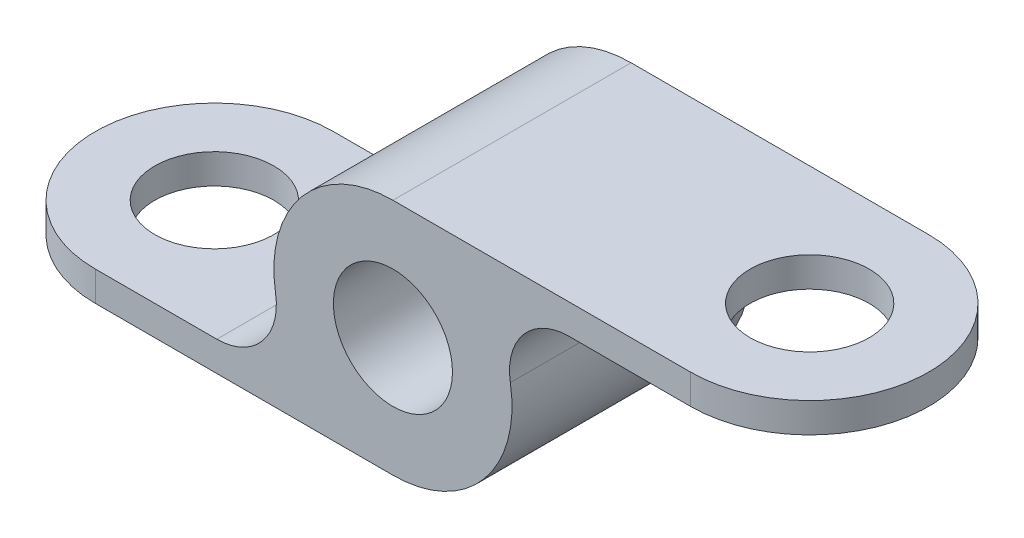
ISO-10303-21;
HEADER;
FILE_DESCRIPTION(('STEP AP214'),'2;1');
FILE_NAME('part.step','',(''),(''),'','','');
FILE_SCHEMA(('AUTOMOTIVE_DESIGN { 1 0 10303 214 1 1 1 1 }'));
ENDSEC;
DATA;
#1=APPLICATION_CONTEXT('core data for automotive mechanical design processes');
#2=APPLICATION_PROTOCOL_DEFINITION('international standard','automotive_design',2000,#1);
#3=PRODUCT_CONTEXT('',#1,'mechanical');
#4=PRODUCT('Part','Part','',(#3));
#5=PRODUCT_RELATED_PRODUCT_CATEGORY('part','',(#4));
#6=PRODUCT_DEFINITION_FORMATION('','',#4);
#7=PRODUCT_DEFINITION_CONTEXT('part definition',#1,'design');
#8=PRODUCT_DEFINITION('design','',#6,#7);
#9=PRODUCT_DEFINITION_SHAPE('','',#8);
#10=(LENGTH_UNIT() NAMED_UNIT(*) SI_UNIT(.MILLI.,.METRE.));
#11=(NAMED_UNIT(*) PLANE_ANGLE_UNIT() SI_UNIT($,.RADIAN.));
#12=(NAMED_UNIT(*) SI_UNIT($,.STERADIAN.) SOLID_ANGLE_UNIT());
#13=UNCERTAINTY_MEASURE_WITH_UNIT(LENGTH_MEASURE(1.E-05),#10,'distance_accuracy_value','');
#14=(GEOMETRIC_REPRESENTATION_CONTEXT(3) GLOBAL_UNCERTAINTY_ASSIGNED_CONTEXT((#13)) GLOBAL_UNIT_ASSIGNED_CONTEXT((#10,
#11,#12)) REPRESENTATION_CONTEXT('',''));
#15=CARTESIAN_POINT('',(0.,0.,0.));
#16=DIRECTION('',(0.,0.,1.));
#17=DIRECTION('',(1.,0.,0.));
#18=AXIS2_PLACEMENT_3D('',#15,#16,#17);
#19=CARTESIAN_POINT('',(0.,0.,20.));
#20=DIRECTION('',(0.,0.,-1.));
#21=DIRECTION('',(-1.,0.,0.));
#22=AXIS2_PLACEMENT_3D('',#19,#20,#21);
#23=CYLINDRICAL_SURFACE('',#22,10.);
#24=CARTESIAN_POINT('',(0.,0.,0.));
#25=DIRECTION('',(0.,0.,1.));
#26=DIRECTION('',(1.,0.,0.));
#27=AXIS2_PLACEMENT_3D('',#24,#25,#26);
#28=CIRCLE('',#27,10.);
#29=CARTESIAN_POINT('',(0.,-10.,0.));
#30=VERTEX_POINT('',#29);
#31=CARTESIAN_POINT('',(9.8601329718327,1.66666666666667,0.));
#32=VERTEX_POINT('',#31);
#33=EDGE_CURVE('E163',#30,#32,#28,.T.);
#34=ORIENTED_EDGE('',*,*,#33,.T.);
#35=DIRECTION('',(0.,0.,1.));
#36=VECTOR('',#35,1.);
#37=CARTESIAN_POINT('',(9.8601329718327,1.66666666666667,0.));
#38=LINE('',#37,#36);
#39=CARTESIAN_POINT('',(9.8601329718327,1.66666666666667,20.));
#40=VERTEX_POINT('',#39);
#41=EDGE_CURVE('E179',#32,#40,#38,.T.);
#42=ORIENTED_EDGE('',*,*,#41,.T.);
#43=CARTESIAN_POINT('',(0.,0.,20.));
#44=DIRECTION('',(0.,0.,1.));
#45=DIRECTION('',(1.,0.,0.));
#46=AXIS2_PLACEMENT_3D('',#43,#44,#45);
#47=CIRCLE('',#46,10.);
#48=CARTESIAN_POINT('',(0.,-10.,20.));
#49=VERTEX_POINT('',#48);
#50=EDGE_CURVE('E57',#49,#40,#47,.T.);
#51=ORIENTED_EDGE('',*,*,#50,.F.);
#52=DIRECTION('',(0.,0.,1.));
#53=VECTOR('',#52,1.);
#54=CARTESIAN_POINT('',(0.,-10.,0.));
#55=LINE('',#54,#53);
#56=EDGE_CURVE('E157',#30,#49,#55,.T.);
#57=ORIENTED_EDGE('',*,*,#56,.F.);
#58=EDGE_LOOP('',(#34,#42,#51,#57));
#59=FACE_BOUND('',#58,.T.);
#60=ADVANCED_FACE('F50',(#59),#23,.T.);
#61=CARTESIAN_POINT('',(0.,10.,0.));
#62=VERTEX_POINT('',#61);
#63=CARTESIAN_POINT('',(-9.8601329718327,-1.66666666666667,0.));
#64=VERTEX_POINT('',#63);
#65=EDGE_CURVE('E51',#62,#64,#28,.T.);
#66=ORIENTED_EDGE('',*,*,#65,.T.);
#67=DIRECTION('',(0.,0.,1.));
#68=VECTOR('',#67,1.);
#69=CARTESIAN_POINT('',(-9.8601329718327,-1.66666666666667,0.));
#70=LINE('',#69,#68);
#71=CARTESIAN_POINT('',(-9.8601329718327,-1.66666666666667,20.));
#72=VERTEX_POINT('',#71);
#73=EDGE_CURVE('E191',#64,#72,#70,.T.);
#74=ORIENTED_EDGE('',*,*,#73,.T.);
#75=CARTESIAN_POINT('',(0.,10.,20.));
#76=VERTEX_POINT('',#75);
#77=EDGE_CURVE('E11',#76,#72,#47,.T.);
#78=ORIENTED_EDGE('',*,*,#77,.F.);
#79=DIRECTION('',(0.,0.,1.));
#80=VECTOR('',#79,1.);
#81=CARTESIAN_POINT('',(0.,10.,0.));
#82=LINE('',#81,#80);
#83=EDGE_CURVE('E148',#62,#76,#82,.T.);
#84=ORIENTED_EDGE('',*,*,#83,.F.);
#85=EDGE_LOOP('',(#66,#74,#78,#84));
#86=FACE_BOUND('',#85,.T.);
#87=ADVANCED_FACE('F47',(#86),#23,.T.);
#88=CARTESIAN_POINT('',(0.,0.,20.));
#89=DIRECTION('',(0.,0.,1.));
#90=DIRECTION('',(1.,0.,0.));
#91=AXIS2_PLACEMENT_3D('',#88,#89,#90);
#92=PLANE('',#91);
#93=CARTESIAN_POINT('',(0.,0.,20.));
#94=DIRECTION('',(0.,0.,1.));
#95=DIRECTION('',(1.,0.,0.));
#96=AXIS2_PLACEMENT_3D('',#93,#94,#95);
#97=CIRCLE('',#96,5.);
#98=CARTESIAN_POINT('',(5.,0.,20.));
#99=VERTEX_POINT('',#98);
#100=EDGE_CURVE('E227',#99,#99,#97,.T.);
#101=ORIENTED_EDGE('',*,*,#100,.F.);
#102=EDGE_LOOP('',(#101));
#103=FACE_BOUND('',#102,.T.);
#104=ORIENTED_EDGE('',*,*,#77,.T.);
#105=CARTESIAN_POINT('',(-14.790199457749,-2.5,20.));
#106=DIRECTION('',(0.,0.,1.));
#107=DIRECTION('',(1.,0.,0.));
#108=AXIS2_PLACEMENT_3D('',#105,#106,#107);
#109=CIRCLE('',#108,5.);
#110=CARTESIAN_POINT('',(-14.790199457749,-7.5,20.));
#111=VERTEX_POINT('',#110);
#112=EDGE_CURVE('E69',#111,#72,#109,.T.);
#113=ORIENTED_EDGE('',*,*,#112,.F.);
#114=DIRECTION('',(-1.,0.,0.));
#115=VECTOR('',#114,1.);
#116=CARTESIAN_POINT('',(-25.,-7.5,20.));
#117=LINE('',#116,#115);
#118=CARTESIAN_POINT('',(-25.,-7.5,20.));
#119=VERTEX_POINT('',#118);
#120=EDGE_CURVE('E194',#111,#119,#117,.T.);
#121=ORIENTED_EDGE('',*,*,#120,.T.);
#122=DIRECTION('',(0.,-1.,0.));
#123=VECTOR('',#122,1.);
#124=CARTESIAN_POINT('',(-25.,-10.,20.));
#125=LINE('',#124,#123);
#126=CARTESIAN_POINT('',(-25.,-10.,20.));
#127=VERTEX_POINT('',#126);
#128=EDGE_CURVE('E192',#119,#127,#125,.T.);
#129=ORIENTED_EDGE('',*,*,#128,.T.);
#130=DIRECTION('',(1.,0.,0.));
#131=VECTOR('',#130,1.);
#132=CARTESIAN_POINT('',(0.,-10.,20.));
#133=LINE('',#132,#131);
#134=EDGE_CURVE('E176',#127,#49,#133,.T.);
#135=ORIENTED_EDGE('',*,*,#134,.T.);
#136=ORIENTED_EDGE('',*,*,#50,.T.);
#137=CARTESIAN_POINT('',(14.790199457749,2.5,20.));
#138=DIRECTION('',(0.,0.,1.));
#139=DIRECTION('',(1.,0.,0.));
#140=AXIS2_PLACEMENT_3D('',#137,#138,#139);
#141=CIRCLE('',#140,5.);
#142=CARTESIAN_POINT('',(14.790199457749,7.5,20.));
#143=VERTEX_POINT('',#142);
#144=EDGE_CURVE('E64',#143,#40,#141,.T.);
#145=ORIENTED_EDGE('',*,*,#144,.F.);
#146=DIRECTION('',(1.,0.,0.));
#147=VECTOR('',#146,1.);
#148=CARTESIAN_POINT('',(25.,7.5,20.));
#149=LINE('',#148,#147);
#150=CARTESIAN_POINT('',(25.,7.5,20.));
#151=VERTEX_POINT('',#150);
#152=EDGE_CURVE('E154',#143,#151,#149,.T.);
#153=ORIENTED_EDGE('',*,*,#152,.T.);
#154=DIRECTION('',(0.,1.,0.));
#155=VECTOR('',#154,1.);
#156=CARTESIAN_POINT('',(25.,10.,20.));
#157=LINE('',#156,#155);
#158=CARTESIAN_POINT('',(25.,10.,20.));
#159=VERTEX_POINT('',#158);
#160=EDGE_CURVE('E133',#151,#159,#157,.T.);
#161=ORIENTED_EDGE('',*,*,#160,.T.);
#162=DIRECTION('',(-1.,0.,0.));
#163=VECTOR('',#162,1.);
#164=CARTESIAN_POINT('',(0.,10.,20.));
#165=LINE('',#164,#163);
#166=EDGE_CURVE('E141',#159,#76,#165,.T.);
#167=ORIENTED_EDGE('',*,*,#166,.T.);
#168=EDGE_LOOP('',(#104,#113,#121,#129,#135,#136,#145,#153,#161,#167));
#169=FACE_BOUND('',#168,.T.);
#170=ADVANCED_FACE('F173',(#103,#169),#92,.T.);
#171=CARTESIAN_POINT('',(0.,0.,0.));
#172=DIRECTION('',(0.,0.,1.));
#173=DIRECTION('',(1.,0.,0.));
#174=AXIS2_PLACEMENT_3D('',#171,#172,#173);
#175=PLANE('',#174);
#176=CARTESIAN_POINT('',(0.,0.,0.));
#177=DIRECTION('',(0.,0.,1.));
#178=DIRECTION('',(1.,0.,0.));
#179=AXIS2_PLACEMENT_3D('',#176,#177,#178);
#180=CIRCLE('',#179,5.);
#181=CARTESIAN_POINT('',(5.,0.,0.));
#182=VERTEX_POINT('',#181);
#183=EDGE_CURVE('E221',#182,#182,#180,.T.);
#184=ORIENTED_EDGE('',*,*,#183,.T.);
#185=EDGE_LOOP('',(#184));
#186=FACE_BOUND('',#185,.T.);
#187=ORIENTED_EDGE('',*,*,#65,.F.);
#188=DIRECTION('',(-1.,0.,0.));
#189=VECTOR('',#188,1.);
#190=CARTESIAN_POINT('',(0.,10.,0.));
#191=LINE('',#190,#189);
#192=CARTESIAN_POINT('',(25.,10.,0.));
#193=VERTEX_POINT('',#192);
#194=EDGE_CURVE('E149',#193,#62,#191,.T.);
#195=ORIENTED_EDGE('',*,*,#194,.F.);
#196=DIRECTION('',(0.,1.,0.));
#197=VECTOR('',#196,1.);
#198=CARTESIAN_POINT('',(25.,10.,0.));
#199=LINE('',#198,#197);
#200=CARTESIAN_POINT('',(25.,7.5,0.));
#201=VERTEX_POINT('',#200);
#202=EDGE_CURVE('E129',#201,#193,#199,.T.);
#203=ORIENTED_EDGE('',*,*,#202,.F.);
#204=DIRECTION('',(1.,0.,0.));
#205=VECTOR('',#204,1.);
#206=CARTESIAN_POINT('',(25.,7.5,0.));
#207=LINE('',#206,#205);
#208=CARTESIAN_POINT('',(14.790199457749,7.5,0.));
#209=VERTEX_POINT('',#208);
#210=EDGE_CURVE('E136',#209,#201,#207,.T.);
#211=ORIENTED_EDGE('',*,*,#210,.F.);
#212=CARTESIAN_POINT('',(14.790199457749,2.5,0.));
#213=DIRECTION('',(0.,0.,1.));
#214=DIRECTION('',(1.,0.,0.));
#215=AXIS2_PLACEMENT_3D('',#212,#213,#214);
#216=CIRCLE('',#215,5.);
#217=EDGE_CURVE('E207',#209,#32,#216,.T.);
#218=ORIENTED_EDGE('',*,*,#217,.T.);
#219=ORIENTED_EDGE('',*,*,#33,.F.);
#220=DIRECTION('',(1.,0.,0.));
#221=VECTOR('',#220,1.);
#222=CARTESIAN_POINT('',(0.,-10.,0.));
#223=LINE('',#222,#221);
#224=CARTESIAN_POINT('',(-25.,-10.,0.));
#225=VERTEX_POINT('',#224);
#226=EDGE_CURVE('E184',#225,#30,#223,.T.);
#227=ORIENTED_EDGE('',*,*,#226,.F.);
#228=DIRECTION('',(0.,-1.,0.));
#229=VECTOR('',#228,1.);
#230=CARTESIAN_POINT('',(-25.,-10.,0.));
#231=LINE('',#230,#229);
#232=CARTESIAN_POINT('',(-25.,-7.5,0.));
#233=VERTEX_POINT('',#232);
#234=EDGE_CURVE('E187',#233,#225,#231,.T.);
#235=ORIENTED_EDGE('',*,*,#234,.F.);
#236=DIRECTION('',(-1.,0.,0.));
#237=VECTOR('',#236,1.);
#238=CARTESIAN_POINT('',(-25.,-7.5,0.));
#239=LINE('',#238,#237);
#240=CARTESIAN_POINT('',(-14.790199457749,-7.5,0.));
#241=VERTEX_POINT('',#240);
#242=EDGE_CURVE('E188',#241,#233,#239,.T.);
#243=ORIENTED_EDGE('',*,*,#242,.F.);
#244=CARTESIAN_POINT('',(-14.790199457749,-2.5,0.));
#245=DIRECTION('',(0.,0.,1.));
#246=DIRECTION('',(1.,0.,0.));
#247=AXIS2_PLACEMENT_3D('',#244,#245,#246);
#248=CIRCLE('',#247,5.);
#249=EDGE_CURVE('E202',#241,#64,#248,.T.);
#250=ORIENTED_EDGE('',*,*,#249,.T.);
#251=EDGE_LOOP('',(#187,#195,#203,#211,#218,#219,#227,#235,#243,#250));
#252=FACE_BOUND('',#251,.T.);
#253=ADVANCED_FACE('F147',(#186,#252),#175,.F.);
#254=CARTESIAN_POINT('',(0.,10.,0.));
#255=DIRECTION('',(0.,1.,0.));
#256=DIRECTION('',(0.,0.,1.));
#257=AXIS2_PLACEMENT_3D('',#254,#255,#256);
#258=PLANE('',#257);
#259=CARTESIAN_POINT('',(25.,10.,10.));
#260=DIRECTION('',(0.,1.,0.));
#261=DIRECTION('',(0.,0.,1.));
#262=AXIS2_PLACEMENT_3D('',#259,#260,#261);
#263=CIRCLE('',#262,5.);
#264=CARTESIAN_POINT('',(25.,10.,15.));
#265=VERTEX_POINT('',#264);
#266=EDGE_CURVE('E213',#265,#265,#263,.T.);
#267=ORIENTED_EDGE('',*,*,#266,.F.);
#268=EDGE_LOOP('',(#267));
#269=FACE_BOUND('',#268,.T.);
#270=ORIENTED_EDGE('',*,*,#166,.F.);
#271=CARTESIAN_POINT('',(25.,10.,10.));
#272=DIRECTION('',(0.,1.,0.));
#273=DIRECTION('',(0.,0.,1.));
#274=AXIS2_PLACEMENT_3D('',#271,#272,#273);
#275=CIRCLE('',#274,10.);
#276=EDGE_CURVE('E132',#159,#193,#275,.T.);
#277=ORIENTED_EDGE('',*,*,#276,.T.);
#278=ORIENTED_EDGE('',*,*,#194,.T.);
#279=ORIENTED_EDGE('',*,*,#83,.T.);
#280=EDGE_LOOP('',(#270,#277,#278,#279));
#281=FACE_BOUND('',#280,.T.);
#282=ADVANCED_FACE('F250',(#269,#281),#258,.T.);
#283=CARTESIAN_POINT('',(25.,7.5,0.));
#284=DIRECTION('',(0.,-1.,0.));
#285=DIRECTION('',(0.,0.,-1.));
#286=AXIS2_PLACEMENT_3D('',#283,#284,#285);
#287=PLANE('',#286);
#288=CARTESIAN_POINT('',(25.,7.5,10.));
#289=DIRECTION('',(0.,1.,0.));
#290=DIRECTION('',(0.,0.,1.));
#291=AXIS2_PLACEMENT_3D('',#288,#289,#290);
#292=CIRCLE('',#291,5.);
#293=CARTESIAN_POINT('',(25.,7.5,15.));
#294=VERTEX_POINT('',#293);
#295=EDGE_CURVE('E214',#294,#294,#292,.T.);
#296=ORIENTED_EDGE('',*,*,#295,.T.);
#297=EDGE_LOOP('',(#296));
#298=FACE_BOUND('',#297,.T.);
#299=DIRECTION('',(0.,0.,1.));
#300=VECTOR('',#299,1.);
#301=CARTESIAN_POINT('',(14.790199457749,7.5,0.));
#302=LINE('',#301,#300);
#303=EDGE_CURVE('E142',#209,#143,#302,.T.);
#304=ORIENTED_EDGE('',*,*,#303,.F.);
#305=ORIENTED_EDGE('',*,*,#210,.T.);
#306=CARTESIAN_POINT('',(25.,7.5,10.));
#307=DIRECTION('',(0.,1.,0.));
#308=DIRECTION('',(0.,0.,1.));
#309=AXIS2_PLACEMENT_3D('',#306,#307,#308);
#310=CIRCLE('',#309,10.);
#311=EDGE_CURVE('E121',#151,#201,#310,.T.);
#312=ORIENTED_EDGE('',*,*,#311,.F.);
#313=ORIENTED_EDGE('',*,*,#152,.F.);
#314=EDGE_LOOP('',(#304,#305,#312,#313));
#315=FACE_BOUND('',#314,.T.);
#316=ADVANCED_FACE('F138',(#298,#315),#287,.T.);
#317=CARTESIAN_POINT('',(0.,-10.,0.));
#318=DIRECTION('',(0.,-1.,0.));
#319=DIRECTION('',(0.,0.,-1.));
#320=AXIS2_PLACEMENT_3D('',#317,#318,#319);
#321=PLANE('',#320);
#322=CARTESIAN_POINT('',(-25.,-10.,10.));
#323=DIRECTION('',(0.,-1.,0.));
#324=DIRECTION('',(0.,0.,-1.));
#325=AXIS2_PLACEMENT_3D('',#322,#323,#324);
#326=CIRCLE('',#325,5.);
#327=CARTESIAN_POINT('',(-25.,-10.,5.));
#328=VERTEX_POINT('',#327);
#329=EDGE_CURVE('E222',#328,#328,#326,.T.);
#330=ORIENTED_EDGE('',*,*,#329,.F.);
#331=EDGE_LOOP('',(#330));
#332=FACE_BOUND('',#331,.T.);
#333=ORIENTED_EDGE('',*,*,#134,.F.);
#334=CARTESIAN_POINT('',(-25.,-10.,10.));
#335=DIRECTION('',(0.,-1.,0.));
#336=DIRECTION('',(0.,0.,-1.));
#337=AXIS2_PLACEMENT_3D('',#334,#335,#336);
#338=CIRCLE('',#337,10.);
#339=EDGE_CURVE('E134',#127,#225,#338,.T.);
#340=ORIENTED_EDGE('',*,*,#339,.T.);
#341=ORIENTED_EDGE('',*,*,#226,.T.);
#342=ORIENTED_EDGE('',*,*,#56,.T.);
#343=EDGE_LOOP('',(#333,#340,#341,#342));
#344=FACE_BOUND('',#343,.T.);
#345=ADVANCED_FACE('F185',(#332,#344),#321,.T.);
#346=CARTESIAN_POINT('',(-25.,-7.5,0.));
#347=DIRECTION('',(0.,1.,0.));
#348=DIRECTION('',(0.,0.,1.));
#349=AXIS2_PLACEMENT_3D('',#346,#347,#348);
#350=PLANE('',#349);
#351=CARTESIAN_POINT('',(-25.,-7.5,10.));
#352=DIRECTION('',(0.,-1.,0.));
#353=DIRECTION('',(0.,0.,-1.));
#354=AXIS2_PLACEMENT_3D('',#351,#352,#353);
#355=CIRCLE('',#354,5.);
#356=CARTESIAN_POINT('',(-25.,-7.5,5.));
#357=VERTEX_POINT('',#356);
#358=EDGE_CURVE('E216',#357,#357,#355,.T.);
#359=ORIENTED_EDGE('',*,*,#358,.T.);
#360=EDGE_LOOP('',(#359));
#361=FACE_BOUND('',#360,.T.);
#362=DIRECTION('',(0.,0.,1.));
#363=VECTOR('',#362,1.);
#364=CARTESIAN_POINT('',(-14.790199457749,-7.5,0.));
#365=LINE('',#364,#363);
#366=EDGE_CURVE('E199',#241,#111,#365,.T.);
#367=ORIENTED_EDGE('',*,*,#366,.F.);
#368=ORIENTED_EDGE('',*,*,#242,.T.);
#369=CARTESIAN_POINT('',(-25.,-7.5,10.));
#370=DIRECTION('',(0.,-1.,0.));
#371=DIRECTION('',(0.,0.,-1.));
#372=AXIS2_PLACEMENT_3D('',#369,#370,#371);
#373=CIRCLE('',#372,10.);
#374=EDGE_CURVE('E209',#119,#233,#373,.T.);
#375=ORIENTED_EDGE('',*,*,#374,.F.);
#376=ORIENTED_EDGE('',*,*,#120,.F.);
#377=EDGE_LOOP('',(#367,#368,#375,#376));
#378=FACE_BOUND('',#377,.T.);
#379=ADVANCED_FACE('F294',(#361,#378),#350,.T.);
#380=CARTESIAN_POINT('',(-14.790199457749,-2.5,0.));
#381=DIRECTION('',(0.,0.,1.));
#382=DIRECTION('',(1.,0.,0.));
#383=AXIS2_PLACEMENT_3D('',#380,#381,#382);
#384=CYLINDRICAL_SURFACE('',#383,5.);
#385=ORIENTED_EDGE('',*,*,#112,.T.);
#386=ORIENTED_EDGE('',*,*,#73,.F.);
#387=ORIENTED_EDGE('',*,*,#249,.F.);
#388=ORIENTED_EDGE('',*,*,#366,.T.);
#389=EDGE_LOOP('',(#385,#386,#387,#388));
#390=FACE_BOUND('',#389,.T.);
#391=ADVANCED_FACE('F302',(#390),#384,.F.);
#392=CARTESIAN_POINT('',(14.790199457749,2.5,0.));
#393=DIRECTION('',(0.,0.,1.));
#394=DIRECTION('',(1.,0.,0.));
#395=AXIS2_PLACEMENT_3D('',#392,#393,#394);
#396=CYLINDRICAL_SURFACE('',#395,5.);
#397=ORIENTED_EDGE('',*,*,#144,.T.);
#398=ORIENTED_EDGE('',*,*,#41,.F.);
#399=ORIENTED_EDGE('',*,*,#217,.F.);
#400=ORIENTED_EDGE('',*,*,#303,.T.);
#401=EDGE_LOOP('',(#397,#398,#399,#400));
#402=FACE_BOUND('',#401,.T.);
#403=ADVANCED_FACE('F373',(#402),#396,.F.);
#404=CARTESIAN_POINT('',(-25.,-7.5,10.));
#405=DIRECTION('',(0.,-1.,0.));
#406=DIRECTION('',(0.,0.,-1.));
#407=AXIS2_PLACEMENT_3D('',#404,#405,#406);
#408=CYLINDRICAL_SURFACE('',#407,10.);
#409=ORIENTED_EDGE('',*,*,#339,.F.);
#410=ORIENTED_EDGE('',*,*,#128,.F.);
#411=ORIENTED_EDGE('',*,*,#374,.T.);
#412=ORIENTED_EDGE('',*,*,#234,.T.);
#413=EDGE_LOOP('',(#409,#410,#411,#412));
#414=FACE_BOUND('',#413,.T.);
#415=ADVANCED_FACE('F346',(#414),#408,.T.);
#416=CARTESIAN_POINT('',(25.,7.5,10.));
#417=DIRECTION('',(0.,1.,0.));
#418=DIRECTION('',(0.,0.,1.));
#419=AXIS2_PLACEMENT_3D('',#416,#417,#418);
#420=CYLINDRICAL_SURFACE('',#419,10.);
#421=ORIENTED_EDGE('',*,*,#276,.F.);
#422=ORIENTED_EDGE('',*,*,#160,.F.);
#423=ORIENTED_EDGE('',*,*,#311,.T.);
#424=ORIENTED_EDGE('',*,*,#202,.T.);
#425=EDGE_LOOP('',(#421,#422,#423,#424));
#426=FACE_BOUND('',#425,.T.);
#427=ADVANCED_FACE('F127',(#426),#420,.T.);
#428=CARTESIAN_POINT('',(25.,7.5,10.));
#429=DIRECTION('',(0.,1.,0.));
#430=DIRECTION('',(0.,0.,1.));
#431=AXIS2_PLACEMENT_3D('',#428,#429,#430);
#432=CYLINDRICAL_SURFACE('',#431,5.);
#433=ORIENTED_EDGE('',*,*,#295,.F.);
#434=EDGE_LOOP('',(#433));
#435=FACE_BOUND('',#434,.T.);
#436=ORIENTED_EDGE('',*,*,#266,.T.);
#437=EDGE_LOOP('',(#436));
#438=FACE_BOUND('',#437,.T.);
#439=ADVANCED_FACE('F322',(#435,#438),#432,.F.);
#440=CARTESIAN_POINT('',(-25.,-7.5,10.));
#441=DIRECTION('',(0.,-1.,0.));
#442=DIRECTION('',(0.,0.,-1.));
#443=AXIS2_PLACEMENT_3D('',#440,#441,#442);
#444=CYLINDRICAL_SURFACE('',#443,5.);
#445=ORIENTED_EDGE('',*,*,#358,.F.);
#446=EDGE_LOOP('',(#445));
#447=FACE_BOUND('',#446,.T.);
#448=ORIENTED_EDGE('',*,*,#329,.T.);
#449=EDGE_LOOP('',(#448));
#450=FACE_BOUND('',#449,.T.);
#451=ADVANCED_FACE('F240',(#447,#450),#444,.F.);
#452=CARTESIAN_POINT('',(0.,0.,0.));
#453=DIRECTION('',(0.,0.,1.));
#454=DIRECTION('',(1.,0.,0.));
#455=AXIS2_PLACEMENT_3D('',#452,#453,#454);
#456=CYLINDRICAL_SURFACE('',#455,5.);
#457=ORIENTED_EDGE('',*,*,#183,.F.);
#458=EDGE_LOOP('',(#457));
#459=FACE_BOUND('',#458,.T.);
#460=ORIENTED_EDGE('',*,*,#100,.T.);
#461=EDGE_LOOP('',(#460));
#462=FACE_BOUND('',#461,.T.);
#463=ADVANCED_FACE('F234',(#459,#462),#456,.F.);
#464=CLOSED_SHELL('',(#60,#87,#170,#253,#282,#316,#345,#379,#391,#403,#415,#427,#439,#451,#463));
#465=MANIFOLD_SOLID_BREP('B2',#464);
#466=ADVANCED_BREP_SHAPE_REPRESENTATION('',(#18,#465),#14);
#467=SHAPE_DEFINITION_REPRESENTATION(#9,#466);
ENDSEC;
END-ISO-10303-21;
